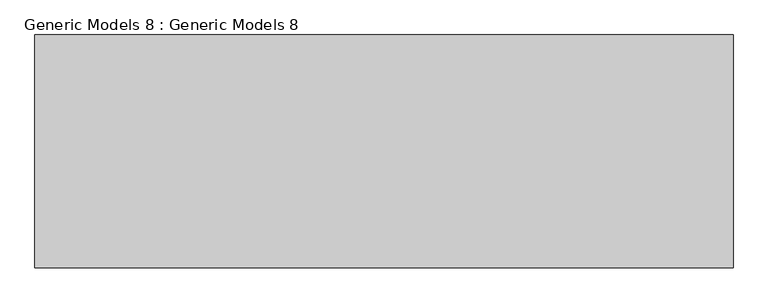
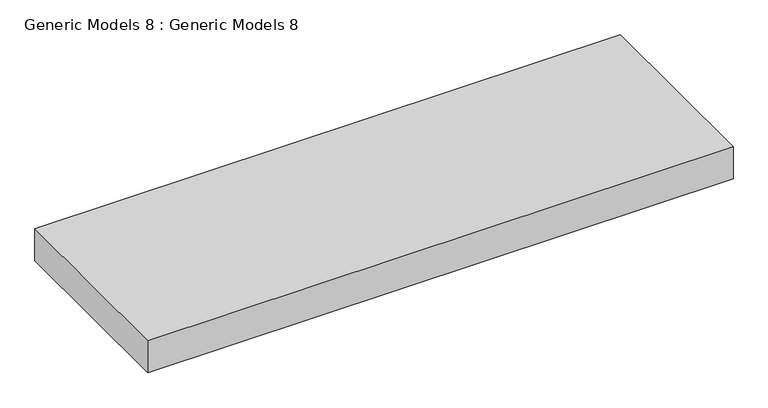
"""IFC4 building model written with IfcOpenShell, lengths in millimetres: proxy geometry, Generic Models 8 : Generic Models 8."""

from ifc_helpers import new_model, si_unit, frame, origin, place, context, project, spatial, polyline, outline, extrude, source, transform, mapped, element, save


def generic_models_8_generic_models_8_c95dbc8d(model_context):
    return source(origin(), model_context, "Body", "SweptSolid", [
        extrude(outline(polyline([(-16665.4247332, 792.9828688), (-16665.4247332, 1679.2875489), (-14009.7161422, 1679.2875489), (-14009.7161422, 792.9828688), (-16665.4247332, 792.9828688)])), frame((0.0, 0.0, 2530.6098734), z_axis=(0.0, 0.0, 1.0), x_axis=(1.0, 0.0, 0.0)), (0.0, 0.0, 1.0), 152.4),
    ])


if __name__ == "__main__":
    model = new_model("IFC4")
    model_context = context("Model", 3, world=origin())
    ifc_project = project(units=[si_unit("LENGTHUNIT", "METRE", prefix="MILLI")], contexts=[model_context])
    site = spatial("IfcSite", under=ifc_project)
    building = spatial("IfcBuilding", under=site)
    placement = place(None, origin())
    generic_models_8_generic_models_8_shape = generic_models_8_generic_models_8_c95dbc8d(model_context)
    element("IfcBuildingElementProxy", 1, Name="Generic Models 8 : Generic Models 8", ObjectType="Generic Models 8 : Generic Models 8", at=placement, inside=building, context=model_context, shape_type="MappedRepresentation", body=[
        mapped(generic_models_8_generic_models_8_shape, transform((0.0, 0.0, 0.0), x_axis=(1.0, 0.0, 0.0), y_axis=(0.0, 1.0, 0.0), z_axis=(0.0, 0.0, 1.0))),
    ])
    save(model, "model.ifc")
